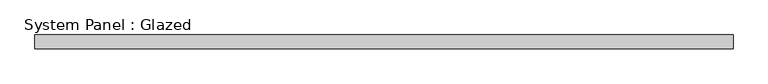
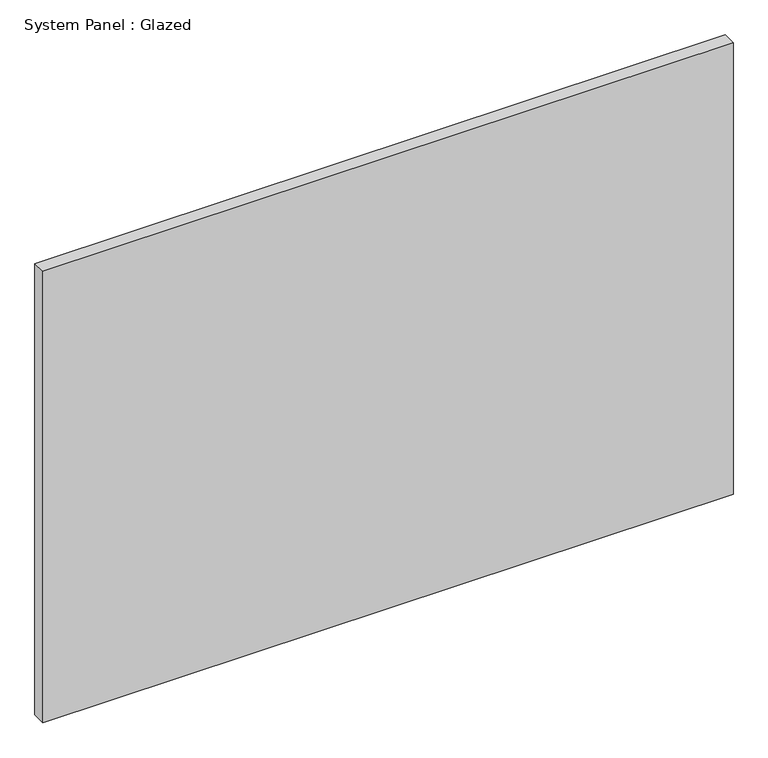
"""IFC4 building model written with IfcOpenShell, lengths in millimetres: plate geometry, System Panel : Glazed."""

from ifc_helpers import new_model, si_unit, origin, origin_with_axes, place, context, project, spatial, polyline, outline, extrude, source, transform, mapped, element, save


def system_panel_glazed_4373b602(model_context):
    return source(origin(), model_context, "Body", "SweptSolid", [
        extrude(outline(polyline([(644.525, 19.05), (-644.525, 19.05), (-644.525, 44.45), (644.525, 44.45), (644.525, 19.05)])), origin_with_axes(), (0.0, 0.0, 1.0), 890.928642),
    ])


if __name__ == "__main__":
    model = new_model("IFC4")
    model_context = context("Model", 3, world=origin())
    ifc_project = project(units=[si_unit("LENGTHUNIT", "METRE", prefix="MILLI")], contexts=[model_context])
    site = spatial("IfcSite", under=ifc_project)
    building = spatial("IfcBuilding", under=site)
    placement = place(None, origin())
    system_panel_glazed_shape = system_panel_glazed_4373b602(model_context)
    element("IfcPlate", 1, ObjectType="System Panel : Glazed", at=placement, inside=building, context=model_context, shape_type="MappedRepresentation", body=[
        mapped(system_panel_glazed_shape, transform((0.0, 0.0, 0.0), x_axis=(1.0, 0.0, 0.0), y_axis=(0.0, 1.0, 0.0), z_axis=(0.0, 0.0, 1.0))),
    ])
    save(model, "model.ifc")

# Revit data of these elements
# Type "System Panel : Glazed"
#   Construction Type Id = "GSP4R"
#   Analytic Construction = "1/8 in Pilkington single glazing"
#   Visual Light Transmittance = 0.9
#   Solar Heat Gain Coefficient = 0.86
#   Heat Transfer Coefficient (U) = 1.18115 BTU/(h·ft²·°F)
#   Define Thermal Properties by = 1
# Element 1 (IfcPlate, "System Panel : Glazed")
#   Materials on its faces: "Glass"
# Materials
#   "Glass": class "Glass", colour RGB 0 128 192, transparency 0.75, Description = "Soda Lime Glass", Cost = 0
